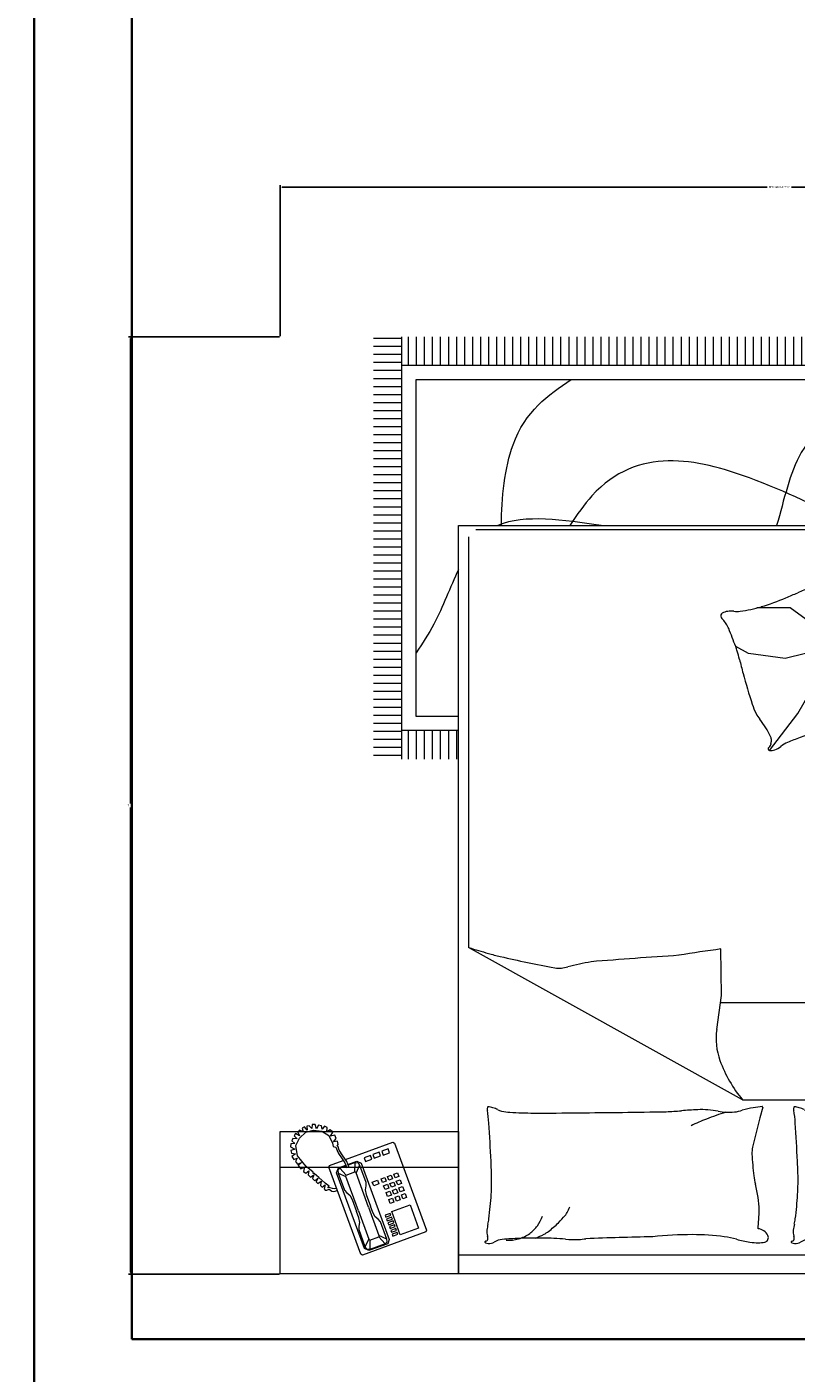
# Model space of a CAD drawing. Units: inches. Extents: x 503 to 1084, y -605 to 132.
# Tile 3 of 14: x 649 to 720, y -437 to -313. Entities that reach past the tile are written whole.
import ezdxf

# ---------------------------------------------------------------- set-up
doc = ezdxf.new("R2010")
doc.units = ezdxf.units.IN
doc.header["$MEASUREMENT"] = 0
doc.layers.add('A-ANNO-DIMS', color=7, linetype='Continuous', lineweight=18)
doc.layers.add('wall', color=1, linetype='Continuous', lineweight=35)
doc.layers.add('furniture', color=50, linetype='Continuous', lineweight=13, transparency=0.8)
doc.styles.add('DIM_FONT', font='SIMPLEX.shx', dxfattribs={"width": 0.8})
doc.styles.get("Standard").update_dxf_attribs({"font": 'arial.ttf'})
doc.dimstyles.get("Standard").update_dxf_attribs({"dimtxt": 0.18, "dimasz": 0.18, "dimexe": 0.18, "dimexo": 0.0625, "dimgap": 0.09, "dimtad": 0, "dimtih": 1, "dimtoh": 1, "dimdec": 1, "dimzin": 0, "dimdsep": 46, "dimlunit": 4, "dimtxsty": 'Standard', "dimcen": 0.09, "dimadec": 0, "dimazin": 0, "dimtfac": 1, "dimtdec": 1, "dimtofl": 0, "dimtmove": 0, "dimatfit": 3, "dimfxl": 1, "dimtolj": 1, "dimtzin": 0, "dimarcsym": 0})

# ---------------------------------------------------------------- blocks, each defined once
blk = doc.blocks.new('A$C4F634EDD')
for p, q in [((0, 2.6295), (0, 2.2295)), ((0.5, 2.6295), (0, 2.6295)), ((0.5, 2.6295), (2.3, 2.6295)), ((0.5, 0.5295), (0.5, 2.6295)), ((0.5, 2.2295), (0.5, 2.6295)), ((2.3, 2.6295), (2.3, 0.5295)), ((2.3, 2.6295), (2.8, 2.6295)), ((2.3, 2.2295), (2.3, 2.6295)), ((2.8, 2.6295), (2.8, 2.2295)), ((0.2457, 2.5697), (0.2457, 2.4733)), ((0.5, 2.5771), (2.3, 2.5771)), ((2.392, 2.5115), (2.5692, 2.5765)), ((2.5692, 2.5765), (2.574, 2.5743)), ((2.574, 2.5743), (2.6638, 2.3298)), ((2.4946, 2.5331), (2.4985, 2.5445)), ((2.5734, 2.3187), (2.4946, 2.5331)), ((2.4985, 2.5445), (2.5516, 2.564)), ((2.5062, 2.5454), (2.5004, 2.5392)), ((2.5004, 2.5392), (2.5013, 2.5315)), ((2.5013, 2.5315), (2.5188, 2.4836)), ((2.5013, 2.5315), (2.5231, 2.5214)), ((2.5062, 2.5454), (2.5487, 2.561)), ((2.5235, 2.5256), (2.5062, 2.5454)), ((2.5483, 2.5347), (2.5235, 2.5256)), ((2.5483, 2.5347), (2.5487, 2.561)), ((2.5514, 2.5318), (2.5483, 2.5347)), ((2.5487, 2.561), (2.5571, 2.56)), ((2.5615, 2.5536), (2.5514, 2.5318)), ((2.5807, 2.4521), (2.5514, 2.5318)), ((2.5516, 2.564), (2.5637, 2.5584)), ((2.5571, 2.56), (2.5615, 2.5536)), ((2.5615, 2.5536), (2.5791, 2.5058)), ((2.5637, 2.5584), (2.6418, 2.3458)), ((2.3898, 2.5066), (2.392, 2.5115)), ((2.4795, 2.2621), (2.3898, 2.5066)), ((2.412, 2.5007), (2.4634, 2.5196)), ((2.4361, 2.4352), (2.412, 2.5007)), ((2.4634, 2.5196), (2.4875, 2.454)), ((2.4842, 2.5232), (2.47, 2.518)), ((2.47, 2.518), (2.472, 2.5127)), ((2.472, 2.5127), (2.4862, 2.5179)), ((2.4881, 2.5126), (2.4739, 2.5074)), ((2.4739, 2.5074), (2.4759, 2.502)), ((2.4759, 2.502), (2.4901, 2.5073)), ((2.492, 2.5019), (2.4778, 2.4967)), ((2.4778, 2.4967), (2.4798, 2.4914)), ((2.4798, 2.4914), (2.494, 2.4966)), ((2.4862, 2.5179), (2.4842, 2.5232)), ((2.4901, 2.5073), (2.4881, 2.5126)), ((2.494, 2.4966), (2.492, 2.5019)), ((2.5231, 2.5214), (2.5235, 2.5256)), ((2.5523, 2.4417), (2.5231, 2.5214)), ((2.5788, 2.4956), (2.5767, 2.4848)), ((2.5791, 2.5058), (2.5788, 2.4956)), ((2.4959, 2.4913), (2.4817, 2.4861)), ((2.4817, 2.4861), (2.4837, 2.4808)), ((2.4837, 2.4808), (2.4979, 2.486)), ((2.4998, 2.4807), (2.4856, 2.4755)), ((2.4856, 2.4755), (2.4876, 2.4702)), ((2.4876, 2.4702), (2.5018, 2.4754)), ((2.5037, 2.47), (2.4895, 2.4648)), ((2.4895, 2.4648), (2.4915, 2.4595)), ((2.4915, 2.4595), (2.5057, 2.4647)), ((2.4979, 2.486), (2.4959, 2.4913)), ((2.5018, 2.4754), (2.4998, 2.4807)), ((2.5057, 2.4647), (2.5037, 2.47)), ((2.5188, 2.4836), (2.5256, 2.4761)), ((2.5256, 2.4761), (2.5342, 2.4692)), ((2.5342, 2.4692), (2.5405, 2.4574)), ((2.5405, 2.4574), (2.547, 2.4397)), ((2.5767, 2.4848), (2.5795, 2.4717)), ((2.5795, 2.4717), (2.586, 2.454)), ((0.0957, 2.4197), (0.192, 2.4197)), ((0.2994, 2.4197), (0.3957, 2.4197)), ((2.4875, 2.454), (2.4361, 2.4352)), ((2.4457, 2.4146), (2.4563, 2.4185)), ((2.4563, 2.4185), (2.4602, 2.4078)), ((2.4634, 2.4211), (2.474, 2.425)), ((2.4673, 2.4104), (2.4634, 2.4211)), ((2.474, 2.425), (2.4779, 2.4143)), ((2.4811, 2.4276), (2.4917, 2.4315)), ((2.485, 2.4169), (2.4811, 2.4276)), ((2.4956, 2.4208), (2.485, 2.4169)), ((2.4917, 2.4315), (2.4956, 2.4208)), ((2.5594, 2.4061), (2.547, 2.4397)), ((2.5523, 2.4417), (2.5875, 2.346)), ((2.5807, 2.4521), (2.6158, 2.3564)), ((2.5984, 2.4204), (2.586, 2.454)), ((2.6047, 2.4086), (2.5984, 2.4204)), ((2.4496, 2.4039), (2.4457, 2.4146)), ((2.4602, 2.4078), (2.4496, 2.4039)), ((2.4528, 2.3951), (2.4635, 2.399)), ((2.4567, 2.3844), (2.4528, 2.3951)), ((2.4674, 2.3883), (2.4567, 2.3844)), ((2.46, 2.3756), (2.4706, 2.3795)), ((2.4635, 2.399), (2.4674, 2.3883)), ((2.4779, 2.4143), (2.4673, 2.4104)), ((2.4706, 2.4016), (2.4812, 2.4055)), ((2.4745, 2.3909), (2.4706, 2.4016)), ((2.4706, 2.3795), (2.4745, 2.3689)), ((2.4851, 2.3949), (2.4745, 2.3909)), ((2.4777, 2.3821), (2.4883, 2.386)), ((2.4816, 2.3715), (2.4777, 2.3821)), ((2.4812, 2.4055), (2.4851, 2.3949)), ((2.4883, 2.4081), (2.4989, 2.412)), ((2.4922, 2.3975), (2.4883, 2.4081)), ((2.4883, 2.386), (2.4922, 2.3754)), ((2.5028, 2.4014), (2.4922, 2.3975)), ((2.4954, 2.3886), (2.5061, 2.3925)), ((2.4993, 2.378), (2.4954, 2.3886)), ((2.4989, 2.412), (2.5028, 2.4014)), ((2.51, 2.3819), (2.4993, 2.378)), ((2.5061, 2.3925), (2.51, 2.3819)), ((2.5238, 2.3769), (2.538, 2.3821)), ((2.538, 2.3821), (2.5419, 2.3715)), ((2.5622, 2.393), (2.5594, 2.4061)), ((2.5598, 2.372), (2.5601, 2.3822)), ((2.5601, 2.3822), (2.5622, 2.393)), ((2.6133, 2.4017), (2.6047, 2.4086)), ((2.6201, 2.3941), (2.6133, 2.4017)), ((2.6376, 2.3463), (2.6201, 2.3941)), ((2.6499, 2.3979), (2.6397, 2.3953)), ((2.6417, 2.39), (2.6488, 2.391)), ((2.6488, 2.391), (2.6538, 2.3895)), ((2.6551, 2.397), (2.6499, 2.3979)), ((2.6538, 2.3895), (2.6596, 2.388)), ((2.6627, 2.392), (2.6551, 2.397)), ((2.6596, 2.388), (2.6626, 2.3867)), ((2.6626, 2.3867), (2.6662, 2.388)), ((2.6692, 2.394), (2.6627, 2.392)), ((2.6662, 2.388), (2.6632, 2.3828)), ((2.6632, 2.3828), (2.6736, 2.3744)), ((2.6736, 2.3944), (2.6692, 2.394)), ((2.6765, 2.391), (2.6736, 2.3944)), ((2.6742, 2.3795), (2.6765, 2.391)), ((2.6824, 2.3858), (2.6742, 2.3795)), ((2.6873, 2.3815), (2.6824, 2.3858)), ((2.6853, 2.369), (2.6873, 2.3815)), ((0.2457, 2.366), (0.2457, 2.2697)), ((2.4639, 2.365), (2.46, 2.3756)), ((2.4745, 2.3689), (2.4639, 2.365)), ((2.4672, 2.3561), (2.4778, 2.36)), ((2.4711, 2.3455), (2.4672, 2.3561)), ((2.4817, 2.3494), (2.4711, 2.3455)), ((2.4778, 2.36), (2.4817, 2.3494)), ((2.4922, 2.3754), (2.4816, 2.3715)), ((2.4849, 2.3626), (2.4955, 2.3665)), ((2.4888, 2.352), (2.4849, 2.3626)), ((2.4994, 2.3559), (2.4888, 2.352)), ((2.4955, 2.3665), (2.4994, 2.3559)), ((2.5026, 2.3691), (2.5132, 2.373)), ((2.5065, 2.3585), (2.5026, 2.3691)), ((2.5171, 2.3624), (2.5065, 2.3585)), ((2.5132, 2.373), (2.5171, 2.3624)), ((2.5277, 2.3663), (2.5238, 2.3769)), ((2.5419, 2.3715), (2.5277, 2.3663)), ((2.5774, 2.3242), (2.5598, 2.372)), ((2.5774, 2.3242), (2.5875, 2.346)), ((2.5875, 2.346), (2.5905, 2.3431)), ((2.5905, 2.3431), (2.5901, 2.3168)), ((2.6154, 2.3522), (2.5905, 2.3431)), ((2.6158, 2.3564), (2.6154, 2.3522)), ((2.6154, 2.3522), (2.6327, 2.3324)), ((2.6376, 2.3463), (2.6158, 2.3564)), ((2.6418, 2.3458), (2.6369, 2.332)), ((2.6385, 2.3386), (2.6376, 2.3463)), ((2.6736, 2.3744), (2.6922, 2.3593)), ((2.6946, 2.376), (2.6853, 2.369)), ((2.6922, 2.3593), (2.7051, 2.3473)), ((2.6995, 2.3713), (2.6946, 2.376)), ((2.695, 2.3603), (2.6995, 2.3713)), ((2.7031, 2.3682), (2.695, 2.3603)), ((2.7096, 2.3616), (2.7031, 2.3682)), ((2.7051, 2.3473), (2.7079, 2.3475)), ((2.7062, 2.351), (2.7096, 2.3616)), ((2.7147, 2.3578), (2.7062, 2.351)), ((2.7079, 2.3475), (2.7079, 2.3443)), ((2.7079, 2.3443), (2.727, 2.3277)), ((2.7214, 2.3517), (2.7147, 2.3578)), ((2.7196, 2.34), (2.7214, 2.3517)), ((2.7286, 2.3466), (2.7196, 2.34)), ((2.7346, 2.3423), (2.7286, 2.3466)), ((2.732, 2.3295), (2.7346, 2.3423)), ((0, 2.3301), (0.5, 2.3301)), ((2.8, 2.3301), (2.3, 2.3301)), ((2.6172, 2.3086), (2.4844, 2.2599)), ((2.5362, 2.305), (2.5185, 2.2985)), ((2.5401, 2.2944), (2.5362, 2.305)), ((2.561, 2.3141), (2.5433, 2.3076)), ((2.5433, 2.3076), (2.5472, 2.297)), ((2.5649, 2.3035), (2.561, 2.3141)), ((2.5855, 2.3131), (2.5734, 2.3187)), ((2.5818, 2.3178), (2.5774, 2.3242)), ((2.5901, 2.3168), (2.5818, 2.3178)), ((2.6104, 2.3222), (2.5855, 2.3131)), ((2.5901, 2.3168), (2.6097, 2.324)), ((2.613, 2.3312), (2.6077, 2.3293)), ((2.6077, 2.3293), (2.6135, 2.3141)), ((2.6192, 2.3174), (2.613, 2.3312)), ((2.6135, 2.3141), (2.6244, 2.2977)), ((2.6153, 2.3261), (2.6327, 2.3324)), ((2.6369, 2.332), (2.6161, 2.3243)), ((2.626, 2.3069), (2.6192, 2.3174)), ((2.6616, 2.3249), (2.6234, 2.3109)), ((2.6365, 2.2916), (2.626, 2.3069)), ((2.6327, 2.3324), (2.6385, 2.3386)), ((2.6638, 2.3298), (2.6616, 2.3249)), ((2.727, 2.3277), (2.7512, 2.2983)), ((2.7423, 2.3345), (2.732, 2.3295)), ((2.7406, 2.3172), (2.7495, 2.325)), ((2.7519, 2.3218), (2.7406, 2.3172)), ((2.7495, 2.325), (2.7423, 2.3345)), ((2.7575, 2.3144), (2.7519, 2.3218)), ((2.7526, 2.3045), (2.7575, 2.3144)), ((2.7622, 2.308), (2.7526, 2.3045)), ((2.7673, 2.2997), (2.7622, 2.308)), ((0.5953, 2.1912), (0.616, 2.2738)), ((1.4546, 2.1912), (1.4752, 2.2738)), ((2.5114, 2.2959), (2.4936, 2.2894)), ((2.4936, 2.2894), (2.4976, 2.2788)), ((2.4976, 2.2788), (2.5153, 2.2853)), ((2.5153, 2.2853), (2.5114, 2.2959)), ((2.5185, 2.2985), (2.5224, 2.2879)), ((2.5224, 2.2879), (2.5401, 2.2944)), ((2.5472, 2.297), (2.5649, 2.3035)), ((2.6244, 2.2977), (2.6349, 2.2825)), ((2.6349, 2.2825), (2.638, 2.273)), ((2.6407, 2.2834), (2.6365, 2.2916)), ((2.6399, 2.2712), (2.6374, 2.2659)), ((2.638, 2.273), (2.6399, 2.2712)), ((2.6438, 2.2739), (2.6407, 2.2834)), ((2.6519, 2.2716), (2.6438, 2.2739)), ((2.6535, 2.2628), (2.6519, 2.2716)), ((2.756, 2.2695), (2.7459, 2.2483)), ((2.7512, 2.2983), (2.756, 2.2695)), ((2.7574, 2.2924), (2.7673, 2.2997)), ((2.7687, 2.2905), (2.7574, 2.2924)), ((2.7587, 2.279), (2.7699, 2.2828)), ((2.7708, 2.2725), (2.7587, 2.279)), ((2.7699, 2.2828), (2.7687, 2.2905)), ((2.7706, 2.2643), (2.7708, 2.2725)), ((0, 2.2295), (0.5, 2.2295)), ((2.8, 2.2295), (2.3, 2.2295)), ((2.4844, 2.2599), (2.4795, 2.2621)), ((2.6374, 2.2659), (2.6398, 2.257)), ((2.6398, 2.257), (2.6509, 2.259)), ((2.6509, 2.259), (2.6431, 2.2492)), ((2.6431, 2.2492), (2.6473, 2.2398)), ((2.6473, 2.2398), (2.6592, 2.2429)), ((2.6592, 2.2429), (2.6521, 2.2314)), ((2.6521, 2.2314), (2.6598, 2.2248)), ((2.6636, 2.2409), (2.6535, 2.2628)), ((2.6598, 2.2248), (2.6697, 2.2309)), ((2.6836, 2.2287), (2.6636, 2.2409)), ((2.6697, 2.2309), (2.6684, 2.219)), ((2.7063, 2.2256), (2.6836, 2.2287)), ((2.7284, 2.2317), (2.7063, 2.2256)), ((2.7459, 2.2483), (2.7284, 2.2317)), ((2.7386, 2.2208), (2.7354, 2.2306)), ((2.7354, 2.2306), (2.7462, 2.2264)), ((2.7509, 2.2314), (2.7459, 2.2418)), ((2.7459, 2.2418), (2.7568, 2.2352)), ((2.7462, 2.2264), (2.7509, 2.2314)), ((2.7529, 2.2505), (2.7645, 2.2498)), ((2.7607, 2.2424), (2.7529, 2.2505)), ((2.7568, 2.2352), (2.7607, 2.2424)), ((2.759, 2.2637), (2.7706, 2.2643)), ((2.7676, 2.2559), (2.759, 2.2637)), ((2.7645, 2.2498), (2.7676, 2.2559)), ((0.5878, 2.1612), (0.5953, 2.1912)), ((1.4471, 2.1612), (1.4546, 2.1912)), ((2.6684, 2.219), (2.6761, 2.2145)), ((2.6761, 2.2145), (2.6821, 2.2237)), ((2.6821, 2.2237), (2.6843, 2.2135)), ((2.6843, 2.2135), (2.6927, 2.2117)), ((2.6927, 2.2117), (2.6986, 2.222)), ((2.6986, 2.222), (2.7019, 2.2098)), ((2.7019, 2.2098), (2.7102, 2.2104)), ((2.7102, 2.2104), (2.7113, 2.2218)), ((2.7113, 2.2218), (2.7192, 2.2137)), ((2.7192, 2.2137), (2.7255, 2.2152)), ((2.7255, 2.2152), (2.7242, 2.2265)), ((2.7242, 2.2265), (2.7324, 2.2165)), ((2.7324, 2.2165), (2.7386, 2.2208)), ((0.5258, 2.121), (0.5258, 0.5617)), ((1.5035, 2.141), (0.5458, 2.141)), ((1.5035, 2.141), (2.2716, 1.7136)), ((1.576, 1.9433), (1.5624, 1.8479)), ((0.5458, 1.8684), (1.5653, 1.8684)), ((1.5624, 1.8479), (1.5641, 1.7178)), ((2.2716, 0.5617), (2.2716, 1.7136)), ((0.2586, 1.1753), (0.3386, 1.1753)), ((0.3386, 0), (0.3386, 1.1852)), ((0.3486, 1.1052), (0.3486, 1.1852)), ((0.3711, 1.1052), (0.3711, 1.1852)), ((0.3936, 1.1052), (0.3936, 1.1852)), ((0.4161, 1.1052), (0.4161, 1.1852)), ((0.4386, 1.1052), (0.4386, 1.1852)), ((0.4611, 1.1052), (0.4611, 1.1852)), ((0.4836, 1.1052), (0.4836, 1.1852)), ((2.3061, 1.1052), (2.3061, 1.1852)), ((2.3286, 1.1052), (2.3286, 1.1852)), ((2.3511, 1.1052), (2.3511, 1.1852)), ((2.3736, 1.1052), (2.3736, 1.1852)), ((2.3961, 1.1052), (2.3961, 1.1852)), ((2.4186, 1.1052), (2.4186, 1.1852)), ((2.4411, 1.1052), (2.4411, 1.1852)), ((2.4588, 1.1852), (2.4588, 0)), ((2.4588, 1.1753), (2.5388, 1.1753)), ((0.2586, 1.1528), (0.3386, 1.1528)), ((1.031, 1.1612), (1.0448, 1.0581)), ((1.4276, 1.1611), (1.3484, 1.0571)), ((2.4588, 1.1528), (2.5388, 1.1528)), ((0.2586, 1.1303), (0.3386, 1.1303)), ((0.2586, 1.1078), (0.3386, 1.1078)), ((0.3386, 1.1052), (0.5, 1.1052)), ((2.3, 1.1052), (2.4588, 1.1052)), ((2.4588, 1.1303), (2.5388, 1.1303)), ((2.4588, 1.1078), (2.5388, 1.1078)), ((0.2586, 1.0853), (0.3386, 1.0853)), ((0.2586, 1.0628), (0.3386, 1.0628)), ((0.3786, 1.0652), (0.5, 1.0652)), ((0.3786, 0.12), (0.3786, 1.0652)), ((1.0448, 1.0581), (1.019, 0.936)), ((1.1784, 0.9702), (1.1586, 1.0591)), ((2.3, 1.0652), (2.4188, 1.0652)), ((2.4188, 1.0652), (2.4188, 0.12)), ((2.4588, 1.0853), (2.5388, 1.0853)), ((2.4588, 1.0628), (2.5388, 1.0628)), ((0.2586, 1.0403), (0.3386, 1.0403)), ((1.3484, 1.0571), (1.2733, 0.9268)), ((2.4588, 1.0403), (2.5388, 1.0403)), ((0.2586, 1.0178), (0.3386, 1.0178)), ((0.2586, 0.9953), (0.3386, 0.9953)), ((0.8108, 1.0151), (0.7868, 1.0117)), ((0.9054, 0.9773), (0.8108, 1.0151)), ((2.4588, 1.0178), (2.5388, 1.0178)), ((2.4588, 0.9953), (2.5388, 0.9953)), ((0.2586, 0.9728), (0.3386, 0.9728)), ((0.2586, 0.9503), (0.3386, 0.9503)), ((0.9743, 0.8845), (0.9054, 0.9773)), ((1.1982, 0.9129), (1.1784, 0.9702)), ((2.4588, 0.9728), (2.5388, 0.9728)), ((2.4588, 0.9503), (2.5388, 0.9503)), ((0.2586, 0.9278), (0.3386, 0.9278)), ((0.8384, 0.9085), (0.7403, 0.8913)), ((0.9072, 0.912), (0.8384, 0.9085)), ((0.9743, 0.8845), (0.9072, 0.912)), ((1.019, 0.936), (0.9743, 0.8845)), ((1.2555, 0.8715), (1.1982, 0.9129)), ((1.2733, 0.9268), (1.2555, 0.8715)), ((2.4588, 0.9278), (2.5388, 0.9278)), ((0.2586, 0.9053), (0.3386, 0.9053)), ((0.2586, 0.8828), (0.3386, 0.8828)), ((0.7403, 0.8913), (0.737, 0.8849)), ((0.9743, 0.8845), (1.0052, 0.802)), ((0.9743, 0.8845), (1.16, 0.8656)), ((1.1973, 0.8853), (1.2203, 0.829)), ((1.2555, 0.8715), (1.2437, 0.7773)), ((1.2555, 0.8715), (1.384, 0.9031)), ((1.2555, 0.8715), (1.3049, 0.8082)), ((1.384, 0.9031), (1.4868, 0.8892)), ((1.4868, 0.8892), (1.5228, 0.8692)), ((2.4588, 0.9053), (2.5388, 0.9053)), ((2.4588, 0.8828), (2.5388, 0.8828)), ((0.2586, 0.8603), (0.3386, 0.8603)), ((0.2586, 0.8378), (0.3386, 0.8378)), ((1.16, 0.8656), (1.2099, 0.8295)), ((2.4588, 0.8603), (2.5388, 0.8603)), ((2.4588, 0.8378), (2.5388, 0.8378)), ((0.2586, 0.8153), (0.3386, 0.8153)), ((1.0052, 0.802), (0.9846, 0.7194)), ((1.2099, 0.8295), (1.222, 0.8209)), ((1.2203, 0.829), (1.2381, 0.7855)), ((1.3049, 0.8082), (1.3701, 0.7608)), ((2.4588, 0.8153), (2.5388, 0.8153)), ((0.2586, 0.7928), (0.3386, 0.7928)), ((0.2586, 0.7703), (0.3386, 0.7703)), ((1.2419, 0.7626), (1.23, 0.668)), ((1.3701, 0.7608), (1.463, 0.7608)), ((2.4588, 0.7928), (2.5388, 0.7928)), ((2.4588, 0.7703), (2.5388, 0.7703)), ((0.2586, 0.7478), (0.3386, 0.7478)), ((0.2586, 0.7253), (0.3386, 0.7253)), ((0.9846, 0.7194), (0.931, 0.6569)), ((2.4588, 0.7478), (2.5388, 0.7478)), ((2.4588, 0.7253), (2.5388, 0.7253)), ((0.2586, 0.7028), (0.3386, 0.7028)), ((0.2586, 0.6803), (0.3386, 0.6803)), ((2.4588, 0.7028), (2.5388, 0.7028)), ((2.4588, 0.6803), (2.5388, 0.6803)), ((0.2586, 0.6578), (0.3386, 0.6578)), ((2.4588, 0.6578), (2.5388, 0.6578)), ((0.2586, 0.6353), (0.3386, 0.6353)), ((0.2586, 0.6128), (0.3386, 0.6128)), ((2.4588, 0.6353), (2.5388, 0.6353)), ((2.4588, 0.6128), (2.5388, 0.6128)), ((0.2586, 0.5903), (0.3386, 0.5903)), ((0.2586, 0.5678), (0.3386, 0.5678)), ((2.4588, 0.5903), (2.5388, 0.5903)), ((2.4588, 0.5678), (2.5388, 0.5678)), ((0.2586, 0.5453), (0.3386, 0.5453)), ((2.3, 0.5295), (0.5, 0.5295)), ((0.5458, 0.5417), (2.2516, 0.5417)), ((2.4588, 0.5453), (2.5388, 0.5453)), ((0.2586, 0.5228), (0.3386, 0.5228)), ((0.2586, 0.5003), (0.3386, 0.5003)), ((2.4588, 0.5228), (2.5388, 0.5228)), ((2.4588, 0.5003), (2.5388, 0.5003)), ((0.2586, 0.4778), (0.3386, 0.4778)), ((0.2586, 0.4553), (0.3386, 0.4553)), ((2.4588, 0.4778), (2.5388, 0.4778)), ((2.4588, 0.4553), (2.5388, 0.4553)), ((0.2586, 0.4328), (0.3386, 0.4328)), ((2.4588, 0.4328), (2.5388, 0.4328)), ((0.2586, 0.4103), (0.3386, 0.4103)), ((0.2586, 0.3878), (0.3386, 0.3878)), ((2.4588, 0.4103), (2.5388, 0.4103)), ((2.4588, 0.3878), (2.5388, 0.3878)), ((0.2586, 0.3653), (0.3386, 0.3653)), ((0.2586, 0.3428), (0.3386, 0.3428)), ((2.4588, 0.3653), (2.5388, 0.3653)), ((2.4588, 0.3428), (2.5388, 0.3428)), ((0.2586, 0.3203), (0.3386, 0.3203)), ((2.4588, 0.3203), (2.5388, 0.3203)), ((0.2586, 0.2978), (0.3386, 0.2978)), ((0.2586, 0.2753), (0.3386, 0.2753)), ((2.4588, 0.2978), (2.5388, 0.2978)), ((2.4588, 0.2753), (2.5388, 0.2753)), ((0.2586, 0.2528), (0.3386, 0.2528)), ((0.2586, 0.2303), (0.3386, 0.2303)), ((2.4588, 0.2528), (2.5388, 0.2528)), ((2.4588, 0.2303), (2.5388, 0.2303)), ((0.2586, 0.2078), (0.3386, 0.2078)), ((2.4588, 0.2078), (2.5388, 0.2078)), ((0.2586, 0.1853), (0.3386, 0.1853)), ((0.2586, 0.1628), (0.3386, 0.1628)), ((2.4588, 0.1853), (2.5388, 0.1853)), ((2.4588, 0.1628), (2.5388, 0.1628)), ((0.2586, 0.1403), (0.3386, 0.1403)), ((0.2586, 0.1178), (0.3386, 0.1178)), ((2.4188, 0.12), (0.3786, 0.12)), ((2.4588, 0.1403), (2.5388, 0.1403)), ((2.4588, 0.1178), (2.5388, 0.1178)), ((0.2586, 0.0953), (0.3386, 0.0953)), ((2.4588, 0.08), (0.3386, 0.08)), ((0.3486, 0), (0.3486, 0.08)), ((0.3711, 0), (0.3711, 0.08)), ((0.3936, 0), (0.3936, 0.08)), ((0.4161, 0), (0.4161, 0.08)), ((0.4386, 0), (0.4386, 0.08)), ((0.4611, 0), (0.4611, 0.08)), ((0.4836, 0), (0.4836, 0.08)), ((0.5061, 0), (0.5061, 0.08)), ((0.5286, 0), (0.5286, 0.08)), ((0.5511, 0), (0.5511, 0.08)), ((0.5736, 0), (0.5736, 0.08)), ((0.5961, 0), (0.5961, 0.08)), ((0.6186, 0), (0.6186, 0.08)), ((0.6411, 0), (0.6411, 0.08)), ((0.6636, 0), (0.6636, 0.08)), ((0.6861, 0), (0.6861, 0.08)), ((0.7086, 0), (0.7086, 0.08)), ((0.7311, 0), (0.7311, 0.08)), ((0.7536, 0), (0.7536, 0.08)), ((0.7761, 0), (0.7761, 0.08)), ((0.7986, 0), (0.7986, 0.08)), ((0.8211, 0), (0.8211, 0.08)), ((0.8436, 0), (0.8436, 0.08)), ((0.8661, 0), (0.8661, 0.08)), ((0.8886, 0), (0.8886, 0.08)), ((0.9111, 0), (0.9111, 0.08)), ((0.9336, 0), (0.9336, 0.08)), ((0.9561, 0), (0.9561, 0.08)), ((0.9786, 0), (0.9786, 0.08)), ((1.0011, 0), (1.0011, 0.08)), ((1.0236, 0), (1.0236, 0.08)), ((1.0461, 0), (1.0461, 0.08)), ((1.0686, 0), (1.0686, 0.08)), ((1.0911, 0), (1.0911, 0.08)), ((1.1136, 0), (1.1136, 0.08)), ((1.1361, 0), (1.1361, 0.08)), ((1.1586, 0), (1.1586, 0.08)), ((1.1811, 0), (1.1811, 0.08)), ((1.2036, 0), (1.2036, 0.08)), ((1.2261, 0), (1.2261, 0.08)), ((1.2486, 0), (1.2486, 0.08)), ((1.2711, 0), (1.2711, 0.08)), ((1.2936, 0), (1.2936, 0.08)), ((1.3161, 0), (1.3161, 0.08)), ((1.3386, 0), (1.3386, 0.08)), ((1.3611, 0), (1.3611, 0.08)), ((1.3836, 0), (1.3836, 0.08)), ((1.4061, 0), (1.4061, 0.08)), ((1.4286, 0), (1.4286, 0.08)), ((1.4511, 0), (1.4511, 0.08)), ((1.4736, 0), (1.4736, 0.08)), ((1.4961, 0), (1.4961, 0.08)), ((1.5186, 0), (1.5186, 0.08)), ((1.5411, 0), (1.5411, 0.08)), ((1.5636, 0), (1.5636, 0.08)), ((1.5861, 0), (1.5861, 0.08)), ((1.6086, 0), (1.6086, 0.08)), ((1.6311, 0), (1.6311, 0.08)), ((1.6536, 0), (1.6536, 0.08)), ((1.6761, 0), (1.6761, 0.08)), ((1.6986, 0), (1.6986, 0.08)), ((1.7211, 0), (1.7211, 0.08)), ((1.7436, 0), (1.7436, 0.08)), ((1.7661, 0), (1.7661, 0.08)), ((1.7886, 0), (1.7886, 0.08)), ((1.8111, 0), (1.8111, 0.08)), ((1.8336, 0), (1.8336, 0.08)), ((1.8561, 0), (1.8561, 0.08)), ((1.8786, 0), (1.8786, 0.08)), ((1.9011, 0), (1.9011, 0.08)), ((1.9236, 0), (1.9236, 0.08)), ((1.9461, 0), (1.9461, 0.08)), ((1.9686, 0), (1.9686, 0.08)), ((1.9911, 0), (1.9911, 0.08)), ((2.0136, 0), (2.0136, 0.08)), ((2.0361, 0), (2.0361, 0.08)), ((2.0586, 0), (2.0586, 0.08)), ((2.0811, 0), (2.0811, 0.08)), ((2.1036, 0), (2.1036, 0.08)), ((2.1261, 0), (2.1261, 0.08)), ((2.1486, 0), (2.1486, 0.08)), ((2.1711, 0), (2.1711, 0.08)), ((2.1936, 0), (2.1936, 0.08)), ((2.2161, 0), (2.2161, 0.08)), ((2.2386, 0), (2.2386, 0.08)), ((2.2611, 0), (2.2611, 0.08)), ((2.2836, 0), (2.2836, 0.08)), ((2.3061, 0), (2.3061, 0.08)), ((2.3286, 0), (2.3286, 0.08)), ((2.3511, 0), (2.3511, 0.08)), ((2.3736, 0), (2.3736, 0.08)), ((2.3961, 0), (2.3961, 0.08)), ((2.4186, 0), (2.4186, 0.08)), ((2.4411, 0), (2.4411, 0.08)), ((2.4588, 0.0953), (2.5388, 0.0953)), ((0.2586, 0.0728), (0.3386, 0.0728)), ((0.2586, 0.0503), (0.3386, 0.0503)), ((2.4588, 0.0728), (2.5388, 0.0728)), ((2.4588, 0.0503), (2.5388, 0.0503)), ((0.2586, 0.0278), (0.3386, 0.0278)), ((0.2586, 0.0053), (0.3386, 0.0053)), ((2.4588, 0.0278), (2.5388, 0.0278)), ((2.4588, 0.0053), (2.5388, 0.0053))]:
    blk.add_line(p, q)
for radius in [0.1222, 0.0865]:
    blk.add_circle((0.2457, 2.4197), radius)
for centre, radius, start, end in [((0.5848, 2.5274), 0.0131, 101.2724, 206.5805), ((0.5999, 2.4516), 0.0904, 90, 101.2724), ((0.5999, 2.3808), 0.1611, 81.5628, 90), ((0.5788, 2.2388), 0.3048, 74.256, 81.5628), ((0.7272, 2.7653), 0.2422, 254.256, 262.4531), ((0.8402, 3.0514), 0.5293, 276.0867, 280.1899), ((1.1602, -8.1346), 10.6675, 90.30153, 91.21582), ((1.1169, 2.2433), 0.2897, 85.1982, 92.5386), ((1.2142, 3.4021), 0.8732, 265.1982, 269.4243), ((1.2995, 2.4357), 0.0992, 105.9352, 126.0864), ((1.2429, 3.3501), 0.8208, 271.9079, 275.2592), ((1.2995, 2.4357), 0.0992, 85.7841, 105.9352), ((1.3132, 2.5864), 0.0539, 275.2592, 300.6513), ((1.3554, 2.5152), 0.0289, 85.6975, 120.6513), ((1.3556, 2.519), 0.0251, 68.2117, 85.6975), ((1.3739, 2.5288), 0.0156, 158.0096, 201.421), ((1.3634, 2.533), 0.00428, 78.1069, 158.0096), ((1.3647, 2.5395), 0.00232, 258.1069, 19.564), ((1.3637, 2.5391), 0.00342, 19.564, 68.2117), ((1.444, 2.5274), 0.0131, 101.2724, 206.5805), ((1.4591, 2.4516), 0.0904, 90, 101.2724), ((1.4591, 2.3808), 0.1611, 81.5628, 90), ((1.438, 2.2388), 0.3048, 74.256, 81.5628), ((1.5865, 2.7653), 0.2422, 254.256, 262.4531), ((1.4785, 15.4878), 12.9656, 271.22425, 272.05324), ((1.97, 2.3805), 0.1524, 92.5386, 100.1899), ((1.9761, 2.2433), 0.2897, 85.1982, 92.5386), ((2.0734, 3.4021), 0.8732, 265.1982, 269.4243), ((2.1588, 2.4357), 0.0992, 105.9352, 126.0864), ((2.1021, 3.3501), 0.8208, 271.9079, 275.2592), ((2.1588, 2.4357), 0.0992, 85.7841, 105.9352), ((2.1724, 2.5864), 0.0539, 275.2592, 300.6513), ((2.2146, 2.5152), 0.0289, 85.6975, 120.6513), ((2.2149, 2.519), 0.0251, 68.2117, 85.6975), ((2.2331, 2.5288), 0.0156, 158.0096, 201.421), ((2.2226, 2.533), 0.00428, 78.1069, 158.0096), ((2.224, 2.5395), 0.00232, 258.1069, 19.564), ((2.2229, 2.5391), 0.00342, 19.564, 68.2117), ((0.6036, 2.5368), 0.0342, 206.5805, 265.5998), ((1.0898, 2.4496), 0.4918, 173.7676, 180), ((0.5368, 2.3783), 0.1399, 45.0976, 62.7964), ((0.7851, 3.2019), 0.6827, 262.4531, 270), ((0.7851, 3.5682), 1.049, 270, 276.0867), ((1.4317, 2.2032), 0.3916, 128.3886, 133.8115), ((1.2362, 2.45), 0.0768, 117.2396, 128.3886), ((1.3082, 2.3102), 0.234, 110.8603, 117.2396), ((1.2204, 4.0232), 1.4943, 269.4243, 271.9079), ((1.2995, 2.4357), 0.0992, 143.8234, 161.5603), ((1.2995, 2.4357), 0.0992, 126.0864, 143.8234), ((1.1177, 2.5413), 0.246, 347.8905, 351.8665), ((1.3288, 2.5111), 0.0328, 351.8665, 21.421), ((1.4628, 2.5368), 0.0342, 206.5805, 265.5998), ((1.949, 2.4496), 0.4918, 173.7676, 180), ((1.6443, 3.2019), 0.6827, 262.4531, 270), ((1.6443, 3.5682), 1.049, 270, 276.0867), ((2.291, 2.2032), 0.3916, 128.3886, 133.8115), ((2.0954, 2.45), 0.0768, 117.2396, 128.3886), ((2.1674, 2.3102), 0.234, 110.8603, 117.2396), ((2.0797, 4.0232), 1.4943, 269.4243, 271.9079), ((2.1588, 2.4357), 0.0992, 143.8234, 161.5603), ((2.1588, 2.4357), 0.0992, 126.0864, 143.8234), ((1.977, 2.5413), 0.246, 347.8905, 351.8665), ((2.1881, 2.5111), 0.0328, 351.8665, 21.421), ((0.5462, 2.4142), 0.0899, 41.4429, 53.7359), ((0.5741, 2.4389), 0.0526, 25.3551, 41.4429), ((0.4851, 2.3967), 0.1511, 21.8149, 25.3551), ((0.5368, 2.3783), 0.1399, 27.3988, 45.0976), ((1.3127, 2.3625), 0.2002, 151.6832, 156.9972), ((1.1799, 2.4341), 0.0493, 140.9651, 151.6832), ((1.3165, 2.3233), 0.2252, 133.8115, 140.9651), ((2.2605, 2.3525), 0.9131, 172.3191, 176.6313), ((1.5522, 2.448), 0.1983, 167.8905, 172.3191), ((2.1719, 2.3625), 0.2002, 151.6832, 156.9972), ((2.0391, 2.4341), 0.0493, 140.9651, 151.6832), ((2.1757, 2.3233), 0.2252, 133.8115, 140.9651), ((3.1198, 2.3525), 0.9131, 172.3191, 176.6313), ((2.4114, 2.448), 0.1983, 167.8905, 172.3191), ((0.8019, 2.4496), 0.204, 180, 189.6844), ((0.4345, 2.3765), 0.2056, 18.7799, 21.8149), ((0.576, 2.4246), 0.0562, 0, 18.7799), ((0.5406, 2.4246), 0.0915, 345.3149, 0), ((0.5368, 2.3783), 0.1399, 16.515, 27.3988), ((0.5368, 2.3783), 0.1399, 5.6311, 16.515), ((1.6611, 2.4496), 0.204, 180, 189.6844), ((1.4703, 2.5637), 0.882, 189.6844, 192.1984), ((2.0266, 2.3663), 0.6787, 176.6313, 181.6331), ((2.3295, 2.5637), 0.882, 189.6844, 192.1984), ((2.8858, 2.3663), 0.6787, 176.6313, 181.6331), ((0.2982, 2.3103), 0.3171, 8.0051, 12.1984), ((-0.0401, 2.2627), 0.6588, 2.6649, 8.0051), ((2.7128, 2.3859), 1.3652, 181.6331, 183.055), ((1.1575, 2.3103), 0.3171, 8.0051, 12.1984), ((0.8191, 2.2627), 0.6588, 2.6649, 8.0051), ((3.5721, 2.3859), 1.3652, 181.6331, 183.055), ((14.9657, 3.0398), 13.6356, 183.05496, 183.50486), ((15.8249, 3.0398), 13.6356, 183.05496, 183.50486), ((0.5503, 2.2902), 0.0677, 345.9548, 2.6649), ((1.4096, 2.2902), 0.0677, 345.9548, 2.6649), ((1.1303, 1.9835), 0.2721, 85.9172, 93.5552), ((1.1455, 2.197), 0.058, 69.3257, 85.9172), ((0.9871, 1.7772), 0.5066, 65.6735, 69.3257), ((0.6058, 0.9338), 1.4323, 63.5015, 65.6735), ((0.473, 2.8815), 0.7387, 289.428, 291.6577), ((0.473, 2.8815), 0.7387, 291.6577, 293.4844), ((0.473, 2.8815), 0.7387, 293.4844, 295.3111), ((1.1054, 1.9358), 0.3126, 57.865, 63.5015), ((0.8841, 1.5835), 0.7286, 54.1737, 57.865), ((1.6762, 2.2258), 0.3212, 183.5049, 189.9984), ((1.3322, 2.8815), 0.7387, 289.428, 291.6577), ((1.3322, 2.8815), 0.7387, 291.6577, 293.4844), ((1.3322, 2.8815), 0.7387, 293.4844, 295.3111), ((2.5355, 2.2258), 0.3212, 183.5049, 189.9984), ((0.5887, 2.1609), 0.000917, 165.9551, 274.0829), ((0.5695, 2.4301), 0.2708, 274.0829, 279.4841), ((0.5763, 2.3896), 0.2297, 279.4841, 287.3864), ((0.6807, 2.0561), 0.1197, 96.4341, 107.3864), ((0.6836, 2.0301), 0.1459, 78.4414, 96.4341), ((0.473, 2.8815), 0.7387, 287.1982, 289.428), ((0.759, 2.3985), 0.2301, 258.4414, 272.7491), ((0.7026, 3.5718), 1.4048, 272.7491, 274.6176), ((0.9136, 0.9591), 1.2165, 92.6096, 94.6176), ((1.2501, -19.8405), 22.0183, 90.37908, 91.01965), ((1.2012, -3.5404), 5.7185, 89.7135, 90.9704), ((1.224, 1.0141), 1.164, 86.426, 89.7135), ((1.2875, 2.0302), 0.1459, 77.131, 86.426), ((1.3099, 2.1283), 0.0453, 62.7159, 77.131), ((1.3658, 2.2367), 0.0767, 242.7159, 253.7788), ((1.3688, 2.247), 0.0875, 253.7788, 262.8796), ((1.3581, 2.1615), 0.00132, 262.8796, 343.3022), ((1.3409, 2.1667), 0.0193, 343.3022, 9.9984), ((1.448, 2.1609), 0.000917, 165.9551, 274.0829), ((1.4288, 2.4301), 0.2708, 274.0829, 279.4841), ((1.4355, 2.3896), 0.2297, 279.4841, 287.3864), ((1.5399, 2.0561), 0.1197, 96.4341, 107.3864), ((1.5429, 2.0301), 0.1459, 78.4414, 96.4341), ((1.3322, 2.8815), 0.7387, 287.1982, 289.428), ((1.6182, 2.3985), 0.2301, 258.4414, 272.7491), ((1.5619, 3.5718), 1.4048, 272.7491, 274.6176), ((1.7729, 0.9591), 1.2165, 92.6096, 94.6176), ((2.1093, -19.8405), 22.0183, 90.37908, 91.01965), ((2.0605, -3.5404), 5.7185, 89.7135, 90.9704), ((2.0833, 1.0141), 1.164, 86.426, 89.7135), ((2.1467, 2.0302), 0.1459, 77.131, 86.426), ((2.1691, 2.1283), 0.0453, 62.7159, 77.131), ((2.2251, 2.2367), 0.0767, 242.7159, 253.7788), ((2.2281, 2.247), 0.0875, 253.7788, 262.8796), ((2.2174, 2.1615), 0.00132, 262.8796, 343.3022), ((2.2001, 2.1667), 0.0193, 343.3022, 9.9984), ((0.5458, 2.121), 0.02, 90, 180), ((1.2147, 1.9017), 0.3751, 20.1488, 39.6445), ((1.3977, 1.9688), 0.1801, 351.8644, 20.1488), ((0.5458, 1.8884), 0.02, 180, 270), ((0.6102, 18.0525), 16.3521, 273.75703, 274.62393), ((1.4194, 4.2174), 2.5158, 281.6741, 283.1904), ((2.0378, 1.5789), 0.1942, 97.7304, 103.1904), ((2.0195, 1.7137), 0.0581, 79.2724, 97.7304), ((1.2737, -2.2227), 4.0646, 77.0745, 79.2724), ((2.0359, 1.0981), 0.6574, 74.0648, 77.0745), ((1.0582, 5.4638), 3.7801, 277.692, 279.495), ((1.7125, -0.0344), 1.8351, 72.2636, 74.0648), ((0.9863, 1.1494), 0.0359, 297.2902, 3.2455), ((1.0348, 1.1521), 0.0127, 51.1864, 183.2455), ((0.9991, 1.1077), 0.0697, 45.8726, 51.1864), ((1.0791, 1.1902), 0.0452, 225.8726, 232.4713), ((1.2846, 1.4577), 0.3825, 232.4713, 233.7837), ((0.6683, 0.6162), 0.6605, 52.7849, 53.7837), ((0.9362, 0.9689), 0.2176, 46.4776, 52.7849), ((1.0543, 1.9106), 0.8371, 290.1287, 292.7069), ((1.3469, 1.2115), 0.0792, 292.7069, 308.5854), ((1.4338, 1.1026), 0.0601, 110.3452, 128.5854), ((1.4251, 1.1259), 0.0352, 86.0516, 110.3452), ((1.4996, 1.1284), 0.0771, 169.5926, 177.2714), ((1.4376, 1.1398), 0.0142, 126.5792, 169.5926), ((1.4273, 1.1567), 0.00443, 13.2808, 86.0516), ((1.4254, 1.1562), 0.0063, 306.5792, 13.2808), ((1.8575, -0.7096), 2.0162, 116.4147, 117.4999), ((-0.4173, 3.8699), 3.0972, 296.4147, 297.2902), ((1.0327, 1.0706), 0.0774, 35.8936, 46.4776), ((1.0771, 1.1027), 0.0226, 351.9508, 35.8936), ((1.1449, 1.0931), 0.0458, 171.9508, 202.4162), ((-0.4107, 5.9078), 5.0942, 289.0836, 290.1287), ((1.4378, 1.1314), 0.0153, 177.2714, 194.5709), ((1.4611, 1.1374), 0.0393, 194.5709, 206.8179), ((1.7401, 1.2785), 0.352, 206.8179, 210.9056), ((1.6045, 1.1973), 0.194, 210.9056, 219.7005), ((-1.8336, 6.2238), 5.8383, 297.49208, 297.84822), ((3.744, -4.3336), 6.1019, 117.49986, 117.84822), ((2.032, 1.4591), 1.0054, 202.4162, 205.0529), ((0.2266, 4.0657), 3.145, 286.6085, 289.0836), ((1.3929, 1.0217), 0.081, 26.0735, 39.7005), ((0.5736, 1.5979), 0.6236, 290.7486, 297.4921), ((1.0922, 1.1636), 0.1166, 280.7366, 286.6085), ((2.6493, 1.7476), 1.6868, 205.0529, 207.0884), ((1.2892, 0.9709), 0.1965, 17.8396, 26.0735), ((-0.4304, 0.4175), 2.003, 15.2625, 17.8396), ((0.6894, 0.9832), 0.0058, 121.6917, 179.0386), ((0.7004, 0.983), 0.0168, 179.0386, 229.4914), ((0.7131, 0.9448), 0.0509, 103.0402, 121.6917), ((0.7152, 0.9361), 0.0599, 86.6119, 103.0402), ((0.7224, 1.0587), 0.063, 266.6119, 282.6252), ((0.6422, 1.4168), 0.43, 282.6252, 290.7486), ((0.6405, 0.9128), 0.0755, 26.3332, 49.4914), ((-1.6775, -0.2344), 2.6619, 25.1732, 26.3332), ((2.541, 1.6922), 1.5652, 207.0884, 209.936), ((-0.0881, 0.5109), 1.6481, 13.841, 15.2625), ((0.9989, 0.8042), 0.2143, 22.2355, 29.936), ((0.5689, 0.8213), 0.1798, 20.7081, 25.1732), ((0.2268, 0.692), 0.5454, 18.2369, 20.7081), ((2.0418, 1.0357), 0.5454, 193.841, 196.3122), ((1.6908, 0.933), 0.1798, 196.3122, 200.7773), ((4.0115, 1.8135), 2.6619, 200.7773, 201.9373), ((2.3102, 1.3785), 1.6481, 198.2369, 199.6584), ((2.6444, 1.4979), 2.003, 199.6584, 202.2355), ((1.6124, 0.8472), 0.0755, 201.9373, 225.0955), ((1.5473, 0.7819), 0.0168, 354.6428, 45.0955), ((1.1727, 0.9313), 0.1794, 277.6784, 284.8807), ((1.2689, 0.569), 0.1955, 97.9822, 104.8807), ((1.2594, 0.7942), 0.0231, 202.2355, 252.8133), ((1.2465, 0.729), 0.034, 85.7407, 97.9822), ((1.2497, 0.772), 0.0092, 265.7407, 289.3799), ((1.2512, 0.7678), 0.00467, 289.3799, 72.8133), ((1.6266, 0.159), 0.6236, 106.3527, 113.0962), ((1.5721, 0.3449), 0.43, 98.2293, 106.3527), ((1.5195, 0.708), 0.063, 82.216, 98.2293), ((1.5362, 0.8298), 0.0599, 262.216, 278.6443), ((1.5375, 0.8209), 0.0509, 278.6443, 297.2959), ((1.5582, 0.7808), 0.0058, 297.2959, 354.6428), ((0.9722, 0.8143), 0.1965, 202.2355, 210.4694), ((2.2689, -2.1899), 3.145, 111.0043, 113.4795), ((0.1831, 0.4093), 1.0054, 18.0203, 19.3448), ((1.0957, 0.7061), 0.0458, 347.5549, 18.0203), ((1.1834, 0.6373), 0.1166, 98.1216, 111.0043), ((1.1763, 0.687), 0.0663, 85.4882, 98.1216), ((1.1871, 0.8241), 0.0712, 265.4882, 277.6784), ((-1.0798, 6.3161), 6.1019, 293.10398, 293.45234), ((3.6722, -4.6377), 5.8383, 113.0962, 113.45234), ((0.8727, 0.7557), 0.081, 210.4694, 224.0964), ((0.6752, 0.5644), 0.194, 35.3015, 44.0964), ((3.0455, -3.9778), 5.0942, 113.4795, 114.5246), ((1.1625, 0.6914), 0.0226, 167.5549, 211.4977), ((2.4404, -2.1823), 3.0972, 112.0188, 112.8944), ((0.5234, 2.5582), 2.0162, 292.0188, 293.104), ((0.5462, 0.4731), 0.352, 31.2138, 35.3015), ((0.8136, 0.6351), 0.0393, 18.9668, 31.2138), ((0.8364, 0.6429), 0.0153, 1.6673, 18.9668), ((0.7746, 0.6411), 0.0771, 353.9885, 1.6673), ((1.2784, -0.1047), 0.8371, 114.5246, 117.1028), ((1.2092, 0.72), 0.0774, 211.4977, 222.0817), ((1.3133, 0.814), 0.2176, 222.0817, 228.389), ((1.6074, 1.1451), 0.6605, 228.389, 229.3878), ((0.9284, 0.3533), 0.3825, 48.0754, 49.3878), ((1.2495, 0.6379), 0.0359, 112.8944, 178.8496), ((0.8506, 0.6191), 0.0063, 130.9751, 197.6767), ((0.8488, 0.6185), 0.00443, 197.6767, 270.4475), ((0.8372, 0.6345), 0.0142, 310.9751, 353.9885), ((0.8486, 0.6493), 0.0352, 270.4475, 294.7411), ((0.8382, 0.6719), 0.0601, 294.7411, 312.9813), ((0.9332, 0.57), 0.0792, 117.1028, 132.9813), ((1.1538, 0.6043), 0.0452, 41.4767, 48.0754), ((1.2399, 0.6804), 0.0697, 221.4767, 226.7905), ((1.2009, 0.6389), 0.0127, 226.7905, 358.8496)]:
    blk.add_arc(centre, radius, start, end)
for points in [[(0.4393, 1.0652), (0.4595, 1.05), (0.4798, 1.0348), (0.5, 1.0195)], [(1.9003, 0.5295), (2.0065, 0.514), (2.1132, 0.4978), (2.1894, 0.5295)]]:
    blk.add_open_spline(points, degree=3)
for points, knots in [([(2.3, 0.6535), (2.3236, 0.7026), (2.3554, 0.7914), (2.4015, 0.8608), (2.4188, 0.8868)], [1893.525221, 1893.525221, 1893.525221, 1893.525221, 2051.902476, 2146.74457, 2146.74457, 2146.74457, 2146.74457]), ([(0.5992, 0.12), (0.6957, 0.2341), (0.8523, 0.4189), (1.0536, 0.5069), (1.136, 0.5295)], [0, 0, 0, 0, 432.822832, 701.445452, 701.445452, 701.445452, 701.445452]), ([(0.7187, 0.12), (0.9791, 0.1362), (1.326, 0.1577), (1.3868, 0.4574), (1.408, 0.5295)], [0, 0, 0, 0, 653.160442, 870.050857, 870.050857, 870.050857, 870.050857]), ([(1.2016, 0.5295), (1.2892, 0.479), (1.5144, 0.3684), (1.8265, 0.2994), (1.9681, 0.4992), (1.9875, 0.5295)], [936.534237, 936.534237, 936.534237, 936.534237, 1243.285375, 1683.261222, 1758.254386, 1758.254386, 1758.254386, 1758.254386]), ([(2.1796, 0.5295), (2.1798, 0.4519), (2.1548, 0.2369), (2.0487, 0.164), (1.9846, 0.12)], [2202.034493, 2202.034493, 2202.034493, 2202.034493, 2357.807635, 2594.446174, 2594.446174, 2594.446174, 2594.446174])]:
    blk.add_open_spline(points, degree=3, knots=knots)
at = {"style": 'DIM_FONT', "width": 0.8, "flags": 9}
for tag, p in [('YSIZE', (0.5, 2.6295)), ('XSIZE', (0.5, 2.6295)), ('XSIZE', (2.2985, 2.6295)), ('YSIZE', (2.2985, 2.6295))]:
    blk.add_attdef(tag, p, '', height=0.0005, dxfattribs=at)
blk = doc.blocks.new('_ArchTick')
at = {"color": 0, "linetype": 'ByBlock', "const_width": 0.15}
blk.add_lwpolyline([(-0.5, -0.5), (0.5, 0.5)], dxfattribs=at)
blk = doc.blocks.new('_Oblique')
at = {"color": 0, "linetype": 'ByBlock', "lineweight": -2}
blk.add_line((-0.5, -0.5), (0.5, 0.5), dxfattribs=at)
blk = doc.blocks.new('*D12')
at = {"layer": 'A-ANNO-DIMS', "color": 0, "lineweight": -2, "transparency": 16777216}
blk.add_line((554.79, -17.82), (554.79, -442.82), dxfattribs=at)
at = {"layer": 'Defpoints', "color": 0, "transparency": 16777216}
for p in [(650.09, -17.82), (554.79, -442.82), (650.09, -442.82)]:
    blk.add_point(p, dxfattribs=at)
at = {"layer": 'A-ANNO-DIMS', "color": 0, "lineweight": -2, "transparency": 16777216, "xscale": 5, "yscale": 5, "zscale": 5}
for name, p, rotation in [('_ArchTick', (554.79, -17.82), 90), ('_Oblique', (554.79, -442.82), 270)]:
    blk.add_blockref(name, p, dxfattribs=dict(at, rotation=rotation))
at = {"layer": 'A-ANNO-DIMS', "color": 0, "transparency": 16777216, "insert": (546.7, -230.32), "char_height": 8, "attachment_point": 5, "rotation": 90}
blk.add_mtext("\\A1;36'", dxfattribs=at)
blk = doc.blocks.new('*D34')
at = {"layer": 'A-ANNO-DIMS', "color": 0, "lineweight": -2, "transparency": 16777216}
for p, q in [((672.72, -341.56), (672.72, -327.68)), ((672.9, -327.86), (717.5, -327.86)), ((764.33, -327.86), (719.73, -327.86)), ((764.51, -341.56), (764.51, -327.68))]:
    blk.add_line(p, q, dxfattribs=at)
at = {"layer": 'A-ANNO-DIMS', "color": 0, "transparency": 16777216}
for points in [[(672.9, -327.83), (672.9, -327.89), (672.72, -327.86)], [(764.33, -327.83), (764.33, -327.89), (764.51, -327.86)]]:
    blk.add_solid(points, dxfattribs=at)
at = {"layer": 'Defpoints', "color": 0, "transparency": 16777216}
for p in [(672.72, -327.86), (672.72, -341.62), (764.51, -341.62)]:
    blk.add_point(p, dxfattribs=at)
at = {"layer": 'A-ANNO-DIMS', "color": 0, "transparency": 16777216, "insert": (718.62, -327.86), "char_height": 0.18, "attachment_point": 5}
blk.add_mtext('\\A1;BED GROUP 7\'-8"', dxfattribs=at)
blk = doc.blocks.new('*D35')
at = {"layer": 'A-ANNO-DIMS', "color": 0, "lineweight": -2, "transparency": 16777216}
for p, q in [((672.66, -341.62), (658.77, -341.62)), ((658.95, -341.8), (658.95, -384.55)), ((658.95, -427.66), (658.95, -384.91)), ((672.66, -427.84), (658.77, -427.84))]:
    blk.add_line(p, q, dxfattribs=at)
at = {"layer": 'A-ANNO-DIMS', "color": 0, "transparency": 16777216}
for points in [[(658.92, -341.8), (658.98, -341.8), (658.95, -341.62)], [(658.92, -427.66), (658.98, -427.66), (658.95, -427.84)]]:
    blk.add_solid(points, dxfattribs=at)
at = {"layer": 'Defpoints', "color": 0, "transparency": 16777216}
for p in [(672.72, -341.62), (658.95, -427.84), (672.72, -427.84)]:
    blk.add_point(p, dxfattribs=at)
at = {"layer": 'A-ANNO-DIMS', "color": 0, "transparency": 16777216, "insert": (658.95, -384.73), "char_height": 0.18, "attachment_point": 5}
blk.add_mtext('\\A1;7\'-2"', dxfattribs=at)

msp = doc.modelspace()

# ---------------------------------------------------------------- linework, layer by layer
at = {"layer": 'wall'}
for p, q in [((650.09, -17.82), (650.09, -514.82)), ((659.09, -26.82), (659.09, -433.82)), ((659.09, -433.82), (779.09, -433.82))]:
    msp.add_line(p, q, dxfattribs=at)

# ---------------------------------------------------------------- block references
at = {"layer": 'furniture', "xscale": 32.78135669785699, "yscale": 32.78135669785699, "zscale": 32.78135669785699, "rotation": 180}
msp.add_blockref('A$C4F634EDD', (764.51, -341.62), dxfattribs=at)

# ---------------------------------------------------------------- dimensions: what is measured, and where the dimension line sits
at = {"layer": 'A-ANNO-DIMS'}
for base, p1, p2, angle, text, override, picture, middle in [((554.79, -442.82), (650.09, -17.82), (650.09, -442.82), 90, "36'", {"dimtxt": 8, "dimasz": 5, "dimgap": 4, "dimtad": 1, "dimtih": 0, "dimblk1": 'ArchTick', "dimblk2": 'Oblique', "dimsah": 1, "dimse1": 1, "dimse2": 1, "dimclrd": 0, "dimclre": 0, "dimclrt": 0}, '*D12', (546.7, -230.32)), ((672.72, -327.86), (764.51, -341.62), (672.72, -341.62), 180, 'BED GROUP <>', {"dimdec": 1, "dimlfac": 1, "dimrnd": 0, "dimzin": 1, "dimdsep": 46, "dimlunit": 4, "dimfrac": 2}, '*D34', (718.62, -327.86))]:
    dim = msp.add_linear_dim(base=base, p1=p1, p2=p2, angle=angle, text=text, dimstyle='Standard', override=override, dxfattribs=at)
    dim.commit()
    dim.dimension.update_dxf_attribs({"geometry": picture, "text_midpoint": middle})
dim = msp.add_linear_dim(base=(658.95, -427.84), p1=(672.72, -341.62), p2=(672.72, -427.84), angle=270, dimstyle='Standard', override={"dimdec": 1, "dimlfac": 1, "dimrnd": 0, "dimzin": 1, "dimdsep": 46, "dimlunit": 4, "dimfrac": 2}, dxfattribs=at)
dim.commit()
dim.dimension.update_dxf_attribs({"geometry": '*D35', "text_midpoint": (658.95, -384.73)})

doc.saveas('drawing.dxf')
